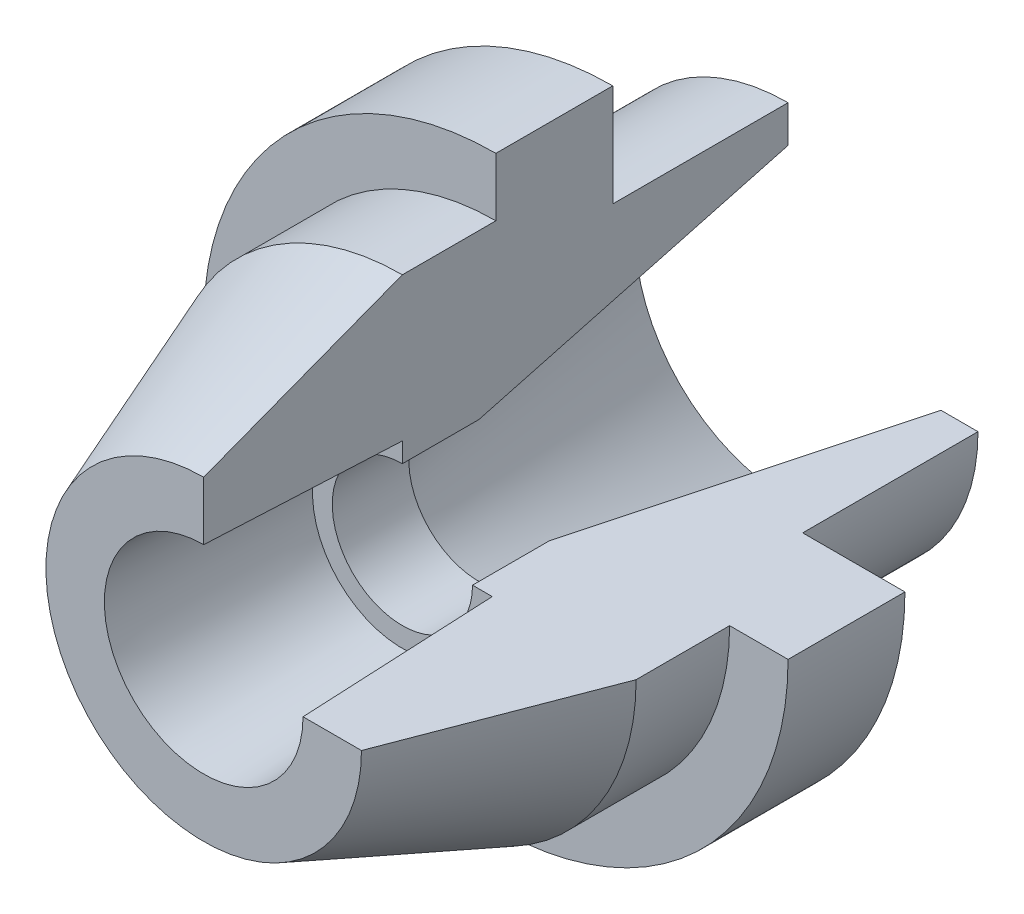
ISO-10303-21;
HEADER;
FILE_DESCRIPTION(('STEP AP214'),'2;1');
FILE_NAME('part.step','',(''),(''),'','','');
FILE_SCHEMA(('AUTOMOTIVE_DESIGN { 1 0 10303 214 1 1 1 1 }'));
ENDSEC;
DATA;
#1=APPLICATION_CONTEXT('core data for automotive mechanical design processes');
#2=APPLICATION_PROTOCOL_DEFINITION('international standard','automotive_design',2000,#1);
#3=PRODUCT_CONTEXT('',#1,'mechanical');
#4=PRODUCT('Part','Part','',(#3));
#5=PRODUCT_RELATED_PRODUCT_CATEGORY('part','',(#4));
#6=PRODUCT_DEFINITION_FORMATION('','',#4);
#7=PRODUCT_DEFINITION_CONTEXT('part definition',#1,'design');
#8=PRODUCT_DEFINITION('design','',#6,#7);
#9=PRODUCT_DEFINITION_SHAPE('','',#8);
#10=(LENGTH_UNIT() NAMED_UNIT(*) SI_UNIT(.MILLI.,.METRE.));
#11=(NAMED_UNIT(*) PLANE_ANGLE_UNIT() SI_UNIT($,.RADIAN.));
#12=(NAMED_UNIT(*) SI_UNIT($,.STERADIAN.) SOLID_ANGLE_UNIT());
#13=UNCERTAINTY_MEASURE_WITH_UNIT(LENGTH_MEASURE(1.E-05),#10,'distance_accuracy_value','');
#14=(GEOMETRIC_REPRESENTATION_CONTEXT(3) GLOBAL_UNCERTAINTY_ASSIGNED_CONTEXT((#13)) GLOBAL_UNIT_ASSIGNED_CONTEXT((#10,
#11,#12)) REPRESENTATION_CONTEXT('',''));
#15=CARTESIAN_POINT('',(0.,0.,0.));
#16=DIRECTION('',(0.,0.,1.));
#17=DIRECTION('',(1.,0.,0.));
#18=AXIS2_PLACEMENT_3D('',#15,#16,#17);
#19=CARTESIAN_POINT('',(0.,0.,0.));
#20=DIRECTION('',(0.,1.,0.));
#21=DIRECTION('',(0.,0.,1.));
#22=AXIS2_PLACEMENT_3D('',#19,#20,#21);
#23=PLANE('',#22);
#24=DIRECTION('',(1.,0.,0.));
#25=VECTOR('',#24,1.);
#26=CARTESIAN_POINT('',(32.5,3.44485451530422E-13,-100.));
#27=LINE('',#26,#25);
#28=CARTESIAN_POINT('',(26.1756249842456,2.78241139488366E-13,-99.9999999999999));
#29=VERTEX_POINT('',#28);
#30=CARTESIAN_POINT('',(32.5,3.44485451530422E-13,-100.));
#31=VERTEX_POINT('',#30);
#32=EDGE_CURVE('E190',#29,#31,#27,.T.);
#33=ORIENTED_EDGE('',*,*,#32,.F.);
#34=DIRECTION('',(0.258819045102517,0.,-0.965925826289069));
#35=VECTOR('',#34,1.);
#36=CARTESIAN_POINT('',(0.,0.,-2.31123763892448));
#37=LINE('',#36,#35);
#38=CARTESIAN_POINT('',(11.9999999999999,0.,-47.0958473297511));
#39=VERTEX_POINT('',#38);
#40=EDGE_CURVE('E268',#29,#39,#37,.F.);
#41=ORIENTED_EDGE('',*,*,#40,.T.);
#42=DIRECTION('',(0.,0.,1.));
#43=VECTOR('',#42,1.);
#44=CARTESIAN_POINT('',(11.9999999999998,1.25693328198351E-13,0.));
#45=LINE('',#44,#43);
#46=CARTESIAN_POINT('',(11.9999999999998,1.27075775336044E-13,-34.));
#47=VERTEX_POINT('',#46);
#48=EDGE_CURVE('E267',#39,#47,#45,.T.);
#49=ORIENTED_EDGE('',*,*,#48,.T.);
#50=DIRECTION('',(1.,0.,0.));
#51=VECTOR('',#50,1.);
#52=CARTESIAN_POINT('',(0.,0.,-34.));
#53=LINE('',#52,#51);
#54=CARTESIAN_POINT('',(15.3800265410508,1.70272611197833E-13,-34.));
#55=VERTEX_POINT('',#54);
#56=EDGE_CURVE('E143',#47,#55,#53,.T.);
#57=ORIENTED_EDGE('',*,*,#56,.T.);
#58=DIRECTION('',(-0.0475922875889132,0.,-0.998866845060969));
#59=VECTOR('',#58,1.);
#60=CARTESIAN_POINT('',(0.,0.,-356.79596897528));
#61=LINE('',#60,#59);
#62=CARTESIAN_POINT('',(17.,1.78065548281E-13,0.));
#63=VERTEX_POINT('',#62);
#64=EDGE_CURVE('E129',#55,#63,#61,.F.);
#65=ORIENTED_EDGE('',*,*,#64,.T.);
#66=DIRECTION('',(-1.,0.,0.));
#67=VECTOR('',#66,1.);
#68=CARTESIAN_POINT('',(0.,0.,0.));
#69=LINE('',#68,#67);
#70=CARTESIAN_POINT('',(27.,2.82809988446294E-13,0.));
#71=VERTEX_POINT('',#70);
#72=EDGE_CURVE('E140',#71,#63,#69,.T.);
#73=ORIENTED_EDGE('',*,*,#72,.F.);
#74=DIRECTION('',(-0.357137466266591,0.,0.934051834851085));
#75=VECTOR('',#74,1.);
#76=CARTESIAN_POINT('',(27.,2.82809988446294E-13,0.));
#77=LINE('',#76,#75);
#78=CARTESIAN_POINT('',(40.,4.2036020779887E-13,-34.));
#79=VERTEX_POINT('',#78);
#80=EDGE_CURVE('E144',#79,#71,#77,.T.);
#81=ORIENTED_EDGE('',*,*,#80,.F.);
#82=DIRECTION('',(0.,0.,1.));
#83=VECTOR('',#82,1.);
#84=CARTESIAN_POINT('',(40.,4.2036020779887E-13,-34.));
#85=LINE('',#84,#83);
#86=CARTESIAN_POINT('',(40.,4.21010771157784E-13,-50.));
#87=VERTEX_POINT('',#86);
#88=EDGE_CURVE('E147',#87,#79,#85,.T.);
#89=ORIENTED_EDGE('',*,*,#88,.F.);
#90=DIRECTION('',(-1.,0.,0.));
#91=VECTOR('',#90,1.);
#92=CARTESIAN_POINT('',(40.,4.21010771157784E-13,-50.));
#93=LINE('',#92,#91);
#94=CARTESIAN_POINT('',(50.,5.25755211323078E-13,-50.));
#95=VERTEX_POINT('',#94);
#96=EDGE_CURVE('E201',#95,#87,#93,.T.);
#97=ORIENTED_EDGE('',*,*,#96,.F.);
#98=DIRECTION('',(0.,0.,1.));
#99=VECTOR('',#98,1.);
#100=CARTESIAN_POINT('',(50.,5.25755211323078E-13,-50.));
#101=LINE('',#100,#99);
#102=CARTESIAN_POINT('',(50.,5.26568415521722E-13,-70.));
#103=VERTEX_POINT('',#102);
#104=EDGE_CURVE('E199',#103,#95,#101,.T.);
#105=ORIENTED_EDGE('',*,*,#104,.F.);
#106=DIRECTION('',(1.,0.,0.));
#107=VECTOR('',#106,1.);
#108=CARTESIAN_POINT('',(50.,5.26568415521722E-13,-70.));
#109=LINE('',#108,#107);
#110=CARTESIAN_POINT('',(32.5,3.43265645232457E-13,-70.));
#111=VERTEX_POINT('',#110);
#112=EDGE_CURVE('E197',#111,#103,#109,.T.);
#113=ORIENTED_EDGE('',*,*,#112,.F.);
#114=DIRECTION('',(0.,0.,1.));
#115=VECTOR('',#114,1.);
#116=CARTESIAN_POINT('',(32.5,3.43265645232457E-13,-70.));
#117=LINE('',#116,#115);
#118=EDGE_CURVE('E186',#31,#111,#117,.T.);
#119=ORIENTED_EDGE('',*,*,#118,.F.);
#120=EDGE_LOOP('',(#33,#41,#49,#57,#65,#73,#81,#89,#97,#105,#113,#119));
#121=FACE_BOUND('',#120,.T.);
#122=ADVANCED_FACE('F39',(#121),#23,.T.);
#123=CARTESIAN_POINT('',(0.,0.,0.));
#124=DIRECTION('',(-1.,0.,0.));
#125=DIRECTION('',(0.,0.,1.));
#126=AXIS2_PLACEMENT_3D('',#123,#124,#125);
#127=PLANE('',#126);
#128=DIRECTION('',(0.,0.258819045102514,-0.96592582628907));
#129=VECTOR('',#128,1.);
#130=CARTESIAN_POINT('',(0.,2.76273577546685E-13,-2.31123763892448));
#131=LINE('',#130,#129);
#132=CARTESIAN_POINT('',(0.,26.1756249842456,-100.));
#133=VERTEX_POINT('',#132);
#134=CARTESIAN_POINT('',(0.,12.,-47.0958473297511));
#135=VERTEX_POINT('',#134);
#136=EDGE_CURVE('E11',#133,#135,#131,.F.);
#137=ORIENTED_EDGE('',*,*,#136,.F.);
#138=DIRECTION('',(0.,1.,0.));
#139=VECTOR('',#138,1.);
#140=CARTESIAN_POINT('',(0.,32.5,-100.));
#141=LINE('',#140,#139);
#142=CARTESIAN_POINT('',(0.,32.5,-100.));
#143=VERTEX_POINT('',#142);
#144=EDGE_CURVE('E266',#133,#143,#141,.T.);
#145=ORIENTED_EDGE('',*,*,#144,.T.);
#146=DIRECTION('',(0.,0.,1.));
#147=VECTOR('',#146,1.);
#148=CARTESIAN_POINT('',(0.,32.5,-70.));
#149=LINE('',#148,#147);
#150=CARTESIAN_POINT('',(0.,32.5,-70.));
#151=VERTEX_POINT('',#150);
#152=EDGE_CURVE('E263',#143,#151,#149,.T.);
#153=ORIENTED_EDGE('',*,*,#152,.T.);
#154=DIRECTION('',(0.,1.,0.));
#155=VECTOR('',#154,1.);
#156=CARTESIAN_POINT('',(0.,50.,-70.));
#157=LINE('',#156,#155);
#158=CARTESIAN_POINT('',(0.,50.,-70.));
#159=VERTEX_POINT('',#158);
#160=EDGE_CURVE('E259',#151,#159,#157,.T.);
#161=ORIENTED_EDGE('',*,*,#160,.T.);
#162=DIRECTION('',(0.,0.,1.));
#163=VECTOR('',#162,1.);
#164=CARTESIAN_POINT('',(0.,50.,-50.));
#165=LINE('',#164,#163);
#166=CARTESIAN_POINT('',(0.,50.,-50.));
#167=VERTEX_POINT('',#166);
#168=EDGE_CURVE('E279',#159,#167,#165,.T.);
#169=ORIENTED_EDGE('',*,*,#168,.T.);
#170=DIRECTION('',(0.,-1.,0.));
#171=VECTOR('',#170,1.);
#172=CARTESIAN_POINT('',(0.,40.,-50.));
#173=LINE('',#172,#171);
#174=CARTESIAN_POINT('',(0.,40.,-50.));
#175=VERTEX_POINT('',#174);
#176=EDGE_CURVE('E253',#167,#175,#173,.T.);
#177=ORIENTED_EDGE('',*,*,#176,.T.);
#178=DIRECTION('',(0.,0.,1.));
#179=VECTOR('',#178,1.);
#180=CARTESIAN_POINT('',(0.,40.,-34.));
#181=LINE('',#180,#179);
#182=CARTESIAN_POINT('',(0.,40.,-34.));
#183=VERTEX_POINT('',#182);
#184=EDGE_CURVE('E193',#175,#183,#181,.T.);
#185=ORIENTED_EDGE('',*,*,#184,.T.);
#186=DIRECTION('',(0.,-0.357137466266591,0.934051834851085));
#187=VECTOR('',#186,1.);
#188=CARTESIAN_POINT('',(0.,27.,0.));
#189=LINE('',#188,#187);
#190=CARTESIAN_POINT('',(0.,27.,0.));
#191=VERTEX_POINT('',#190);
#192=EDGE_CURVE('E187',#183,#191,#189,.T.);
#193=ORIENTED_EDGE('',*,*,#192,.T.);
#194=DIRECTION('',(0.,-1.,0.));
#195=VECTOR('',#194,1.);
#196=CARTESIAN_POINT('',(0.,0.,0.));
#197=LINE('',#196,#195);
#198=CARTESIAN_POINT('',(0.,17.0000000000003,0.));
#199=VERTEX_POINT('',#198);
#200=EDGE_CURVE('E181',#191,#199,#197,.T.);
#201=ORIENTED_EDGE('',*,*,#200,.T.);
#202=DIRECTION('',(0.,-0.047592287588916,-0.998866845060969));
#203=VECTOR('',#202,1.);
#204=CARTESIAN_POINT('',(0.,-7.26244650189538E-13,-356.79596897528));
#205=LINE('',#204,#203);
#206=CARTESIAN_POINT('',(0.,15.380026541051,-33.9999999999999));
#207=VERTEX_POINT('',#206);
#208=EDGE_CURVE('E132',#207,#199,#205,.F.);
#209=ORIENTED_EDGE('',*,*,#208,.F.);
#210=DIRECTION('',(0.,1.,0.));
#211=VECTOR('',#210,1.);
#212=CARTESIAN_POINT('',(0.,0.,-34.));
#213=LINE('',#212,#211);
#214=CARTESIAN_POINT('',(0.,12.,-34.));
#215=VERTEX_POINT('',#214);
#216=EDGE_CURVE('E164',#215,#207,#213,.T.);
#217=ORIENTED_EDGE('',*,*,#216,.F.);
#218=DIRECTION('',(0.,0.,1.));
#219=VECTOR('',#218,1.);
#220=CARTESIAN_POINT('',(0.,12.0000000000001,0.));
#221=LINE('',#220,#219);
#222=EDGE_CURVE('E50',#135,#215,#221,.T.);
#223=ORIENTED_EDGE('',*,*,#222,.F.);
#224=EDGE_LOOP('',(#137,#145,#153,#161,#169,#177,#185,#193,#201,#209,#217,#223));
#225=FACE_BOUND('',#224,.T.);
#226=ADVANCED_FACE('F182',(#225),#127,.F.);
#227=CARTESIAN_POINT('',(0.,0.,0.));
#228=DIRECTION('',(0.,0.,1.));
#229=DIRECTION('',(0.,-1.,0.));
#230=AXIS2_PLACEMENT_3D('',#227,#228,#229);
#231=PLANE('',#230);
#232=ORIENTED_EDGE('',*,*,#72,.T.);
#233=CARTESIAN_POINT('',(0.,2.82809988446294E-13,0.));
#234=DIRECTION('',(0.,0.,1.));
#235=DIRECTION('',(0.,-1.,0.));
#236=AXIS2_PLACEMENT_3D('',#233,#234,#235);
#237=CIRCLE('',#236,17.);
#238=EDGE_CURVE('E127',#199,#63,#237,.T.);
#239=ORIENTED_EDGE('',*,*,#238,.F.);
#240=ORIENTED_EDGE('',*,*,#200,.F.);
#241=CARTESIAN_POINT('',(0.,0.,0.));
#242=DIRECTION('',(0.,0.,-1.));
#243=DIRECTION('',(0.,1.,0.));
#244=AXIS2_PLACEMENT_3D('',#241,#242,#243);
#245=CIRCLE('',#244,27.);
#246=EDGE_CURVE('E65',#71,#191,#245,.T.);
#247=ORIENTED_EDGE('',*,*,#246,.F.);
#248=EDGE_LOOP('',(#232,#239,#240,#247));
#249=FACE_BOUND('',#248,.T.);
#250=ADVANCED_FACE('F41',(#249),#231,.T.);
#251=CARTESIAN_POINT('',(0.,0.,-34.));
#252=DIRECTION('',(0.,0.,-1.));
#253=DIRECTION('',(0.,1.,0.));
#254=AXIS2_PLACEMENT_3D('',#251,#252,#253);
#255=CONICAL_SURFACE('',#254,40.,0.365201449788173);
#256=CARTESIAN_POINT('',(0.,0.,-34.));
#257=DIRECTION('',(0.,0.,-1.));
#258=DIRECTION('',(0.,1.,0.));
#259=AXIS2_PLACEMENT_3D('',#256,#257,#258);
#260=CIRCLE('',#259,40.);
#261=EDGE_CURVE('E161',#79,#183,#260,.T.);
#262=ORIENTED_EDGE('',*,*,#261,.F.);
#263=ORIENTED_EDGE('',*,*,#80,.T.);
#264=ORIENTED_EDGE('',*,*,#246,.T.);
#265=ORIENTED_EDGE('',*,*,#192,.F.);
#266=EDGE_LOOP('',(#262,#263,#264,#265));
#267=FACE_BOUND('',#266,.T.);
#268=ADVANCED_FACE('F215',(#267),#255,.T.);
#269=CARTESIAN_POINT('',(0.,0.,-100.));
#270=DIRECTION('',(0.,0.,-1.));
#271=DIRECTION('',(0.,1.,0.));
#272=AXIS2_PLACEMENT_3D('',#269,#270,#271);
#273=CYLINDRICAL_SURFACE('',#272,40.);
#274=CARTESIAN_POINT('',(0.,0.,-50.));
#275=DIRECTION('',(0.,0.,-1.));
#276=DIRECTION('',(0.,1.,0.));
#277=AXIS2_PLACEMENT_3D('',#274,#275,#276);
#278=CIRCLE('',#277,40.);
#279=EDGE_CURVE('E157',#87,#175,#278,.T.);
#280=ORIENTED_EDGE('',*,*,#279,.F.);
#281=ORIENTED_EDGE('',*,*,#88,.T.);
#282=ORIENTED_EDGE('',*,*,#261,.T.);
#283=ORIENTED_EDGE('',*,*,#184,.F.);
#284=EDGE_LOOP('',(#280,#281,#282,#283));
#285=FACE_BOUND('',#284,.T.);
#286=ADVANCED_FACE('F208',(#285),#273,.T.);
#287=CARTESIAN_POINT('',(40.,4.21010771157784E-13,-50.));
#288=DIRECTION('',(0.,0.,1.));
#289=DIRECTION('',(0.,-1.,0.));
#290=AXIS2_PLACEMENT_3D('',#287,#288,#289);
#291=PLANE('',#290);
#292=CARTESIAN_POINT('',(0.,0.,-50.));
#293=DIRECTION('',(0.,0.,-1.));
#294=DIRECTION('',(0.,1.,0.));
#295=AXIS2_PLACEMENT_3D('',#292,#293,#294);
#296=CIRCLE('',#295,50.);
#297=EDGE_CURVE('E160',#95,#167,#296,.T.);
#298=ORIENTED_EDGE('',*,*,#297,.F.);
#299=ORIENTED_EDGE('',*,*,#96,.T.);
#300=ORIENTED_EDGE('',*,*,#279,.T.);
#301=ORIENTED_EDGE('',*,*,#176,.F.);
#302=EDGE_LOOP('',(#298,#299,#300,#301));
#303=FACE_BOUND('',#302,.T.);
#304=ADVANCED_FACE('F220',(#303),#291,.T.);
#305=CARTESIAN_POINT('',(0.,0.,-100.));
#306=DIRECTION('',(0.,0.,-1.));
#307=DIRECTION('',(0.,1.,0.));
#308=AXIS2_PLACEMENT_3D('',#305,#306,#307);
#309=CYLINDRICAL_SURFACE('',#308,50.);
#310=CARTESIAN_POINT('',(0.,0.,-70.));
#311=DIRECTION('',(0.,0.,-1.));
#312=DIRECTION('',(0.,1.,0.));
#313=AXIS2_PLACEMENT_3D('',#310,#311,#312);
#314=CIRCLE('',#313,50.);
#315=EDGE_CURVE('E154',#103,#159,#314,.T.);
#316=ORIENTED_EDGE('',*,*,#315,.F.);
#317=ORIENTED_EDGE('',*,*,#104,.T.);
#318=ORIENTED_EDGE('',*,*,#297,.T.);
#319=ORIENTED_EDGE('',*,*,#168,.F.);
#320=EDGE_LOOP('',(#316,#317,#318,#319));
#321=FACE_BOUND('',#320,.T.);
#322=ADVANCED_FACE('F238',(#321),#309,.T.);
#323=CARTESIAN_POINT('',(50.,5.26568415521722E-13,-70.));
#324=DIRECTION('',(0.,0.,-1.));
#325=DIRECTION('',(0.,1.,0.));
#326=AXIS2_PLACEMENT_3D('',#323,#324,#325);
#327=PLANE('',#326);
#328=CARTESIAN_POINT('',(0.,0.,-70.));
#329=DIRECTION('',(0.,0.,-1.));
#330=DIRECTION('',(0.,1.,0.));
#331=AXIS2_PLACEMENT_3D('',#328,#329,#330);
#332=CIRCLE('',#331,32.5);
#333=EDGE_CURVE('E146',#111,#151,#332,.T.);
#334=ORIENTED_EDGE('',*,*,#333,.F.);
#335=ORIENTED_EDGE('',*,*,#112,.T.);
#336=ORIENTED_EDGE('',*,*,#315,.T.);
#337=ORIENTED_EDGE('',*,*,#160,.F.);
#338=EDGE_LOOP('',(#334,#335,#336,#337));
#339=FACE_BOUND('',#338,.T.);
#340=ADVANCED_FACE('F237',(#339),#327,.T.);
#341=CARTESIAN_POINT('',(0.,0.,-100.));
#342=DIRECTION('',(0.,0.,-1.));
#343=DIRECTION('',(0.,1.,0.));
#344=AXIS2_PLACEMENT_3D('',#341,#342,#343);
#345=CYLINDRICAL_SURFACE('',#344,32.5);
#346=CARTESIAN_POINT('',(0.,0.,-100.));
#347=DIRECTION('',(0.,0.,-1.));
#348=DIRECTION('',(0.,1.,0.));
#349=AXIS2_PLACEMENT_3D('',#346,#347,#348);
#350=CIRCLE('',#349,32.5);
#351=EDGE_CURVE('E145',#31,#143,#350,.T.);
#352=ORIENTED_EDGE('',*,*,#351,.F.);
#353=ORIENTED_EDGE('',*,*,#118,.T.);
#354=ORIENTED_EDGE('',*,*,#333,.T.);
#355=ORIENTED_EDGE('',*,*,#152,.F.);
#356=EDGE_LOOP('',(#352,#353,#354,#355));
#357=FACE_BOUND('',#356,.T.);
#358=ADVANCED_FACE('F232',(#357),#345,.T.);
#359=CARTESIAN_POINT('',(32.5,3.44485451530422E-13,-100.));
#360=DIRECTION('',(0.,0.,-1.));
#361=DIRECTION('',(0.,1.,0.));
#362=AXIS2_PLACEMENT_3D('',#359,#360,#361);
#363=PLANE('',#362);
#364=ORIENTED_EDGE('',*,*,#144,.F.);
#365=CARTESIAN_POINT('',(0.,0.,-99.9999999999999));
#366=DIRECTION('',(0.,0.,1.));
#367=DIRECTION('',(0.,-1.,0.));
#368=AXIS2_PLACEMENT_3D('',#365,#366,#367);
#369=CIRCLE('',#368,26.1756249842456);
#370=EDGE_CURVE('E142',#133,#29,#369,.T.);
#371=ORIENTED_EDGE('',*,*,#370,.T.);
#372=ORIENTED_EDGE('',*,*,#32,.T.);
#373=ORIENTED_EDGE('',*,*,#351,.T.);
#374=EDGE_LOOP('',(#364,#371,#372,#373));
#375=FACE_BOUND('',#374,.T.);
#376=ADVANCED_FACE('F226',(#375),#363,.T.);
#377=CARTESIAN_POINT('',(0.,0.,-99.9999999999999));
#378=DIRECTION('',(0.,0.,-1.));
#379=DIRECTION('',(0.,1.,0.));
#380=AXIS2_PLACEMENT_3D('',#377,#378,#379);
#381=CONICAL_SURFACE('',#380,26.1756249842456,0.261799387799146);
#382=ORIENTED_EDGE('',*,*,#370,.F.);
#383=ORIENTED_EDGE('',*,*,#136,.T.);
#384=CARTESIAN_POINT('',(0.,1.4961822805434E-13,-47.0958473297511));
#385=DIRECTION('',(0.,0.,1.));
#386=DIRECTION('',(0.,-1.,0.));
#387=AXIS2_PLACEMENT_3D('',#384,#385,#386);
#388=CIRCLE('',#387,11.9999999999999);
#389=EDGE_CURVE('E171',#135,#39,#388,.T.);
#390=ORIENTED_EDGE('',*,*,#389,.T.);
#391=ORIENTED_EDGE('',*,*,#40,.F.);
#392=EDGE_LOOP('',(#382,#383,#390,#391));
#393=FACE_BOUND('',#392,.T.);
#394=ADVANCED_FACE('F234',(#393),#381,.F.);
#395=CARTESIAN_POINT('',(0.,2.82809988446294E-13,0.));
#396=DIRECTION('',(0.,0.,1.));
#397=DIRECTION('',(0.,-1.,0.));
#398=AXIS2_PLACEMENT_3D('',#395,#396,#397);
#399=CYLINDRICAL_SURFACE('',#398,11.9999999999998);
#400=ORIENTED_EDGE('',*,*,#389,.F.);
#401=ORIENTED_EDGE('',*,*,#222,.T.);
#402=CARTESIAN_POINT('',(0.,1.86654592374554E-13,-34.));
#403=DIRECTION('',(0.,0.,1.));
#404=DIRECTION('',(0.,-1.,0.));
#405=AXIS2_PLACEMENT_3D('',#402,#403,#404);
#406=CIRCLE('',#405,11.9999999999998);
#407=EDGE_CURVE('E175',#215,#47,#406,.T.);
#408=ORIENTED_EDGE('',*,*,#407,.T.);
#409=ORIENTED_EDGE('',*,*,#48,.F.);
#410=EDGE_LOOP('',(#400,#401,#408,#409));
#411=FACE_BOUND('',#410,.T.);
#412=ADVANCED_FACE('F172',(#411),#399,.F.);
#413=CARTESIAN_POINT('',(0.,12.,-34.));
#414=DIRECTION('',(0.,0.,1.));
#415=DIRECTION('',(0.,-1.,0.));
#416=AXIS2_PLACEMENT_3D('',#413,#414,#415);
#417=PLANE('',#416);
#418=ORIENTED_EDGE('',*,*,#407,.F.);
#419=ORIENTED_EDGE('',*,*,#216,.T.);
#420=CARTESIAN_POINT('',(0.,1.86654592374554E-13,-34.));
#421=DIRECTION('',(0.,0.,1.));
#422=DIRECTION('',(0.,-1.,0.));
#423=AXIS2_PLACEMENT_3D('',#420,#421,#422);
#424=CIRCLE('',#423,15.3800265410508);
#425=EDGE_CURVE('E53',#207,#55,#424,.T.);
#426=ORIENTED_EDGE('',*,*,#425,.T.);
#427=ORIENTED_EDGE('',*,*,#56,.F.);
#428=EDGE_LOOP('',(#418,#419,#426,#427));
#429=FACE_BOUND('',#428,.T.);
#430=ADVANCED_FACE('F180',(#429),#417,.T.);
#431=CARTESIAN_POINT('',(0.,1.86654592374554E-13,-34.));
#432=DIRECTION('',(0.,0.,1.));
#433=DIRECTION('',(0.,-1.,0.));
#434=AXIS2_PLACEMENT_3D('',#431,#432,#433);
#435=CONICAL_SURFACE('',#434,15.3800265410508,0.0476102722195067);
#436=ORIENTED_EDGE('',*,*,#425,.F.);
#437=ORIENTED_EDGE('',*,*,#208,.T.);
#438=ORIENTED_EDGE('',*,*,#238,.T.);
#439=ORIENTED_EDGE('',*,*,#64,.F.);
#440=EDGE_LOOP('',(#436,#437,#438,#439));
#441=FACE_BOUND('',#440,.T.);
#442=ADVANCED_FACE('F126',(#441),#435,.F.);
#443=CLOSED_SHELL('',(#122,#226,#250,#268,#286,#304,#322,#340,#358,#376,#394,#412,#430,#442));
#444=MANIFOLD_SOLID_BREP('B2',#443);
#445=ADVANCED_BREP_SHAPE_REPRESENTATION('',(#18,#444),#14);
#446=SHAPE_DEFINITION_REPRESENTATION(#9,#445);
ENDSEC;
END-ISO-10303-21;
